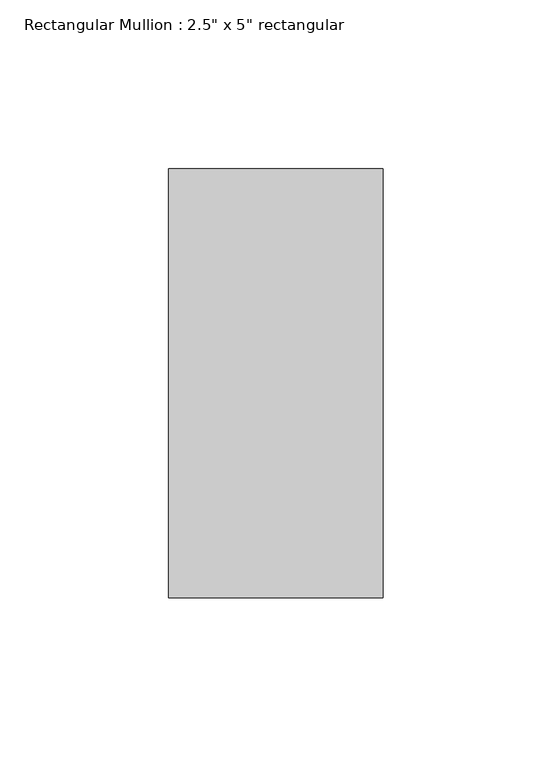
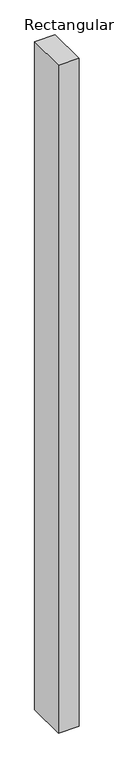
"""IFC4 building model written with IfcOpenShell, lengths in millimetres: member geometry."""

from ifc_helpers import new_model, si_unit, frame, origin, place, context, project, spatial, polyline, outline, extrude, source, transform, mapped, element, save


def member_1ab8d6f1(model_context):
    return source(origin(), model_context, "Body", "SweptSolid", [
        extrude(outline(polyline([(0.0, 63.5), (0.0, -63.5), (-63.5, -63.5), (-63.5, 63.5), (0.0, 63.5)])), frame((0.0, 0.0, -2184.4), z_axis=(0.0, 0.0, 1.0), x_axis=(1.0, 0.0, 0.0)), (0.0, 0.0, 1.0), 2184.4),
    ])


if __name__ == "__main__":
    model = new_model("IFC4")
    model_context = context("Model", 3, world=origin())
    ifc_project = project(units=[si_unit("LENGTHUNIT", "METRE", prefix="MILLI")], contexts=[model_context])
    site = spatial("IfcSite", under=ifc_project)
    building = spatial("IfcBuilding", under=site)
    placement = place(None, origin())
    member_shape = member_1ab8d6f1(model_context)
    element("IfcMember", 1, ObjectType="Rectangular Mullion : 2.5\" x 5\" rectangular", at=placement, inside=building, context=model_context, shape_type="MappedRepresentation", body=[
        mapped(member_shape, transform((0.0, 0.0, 0.0), x_axis=(1.0, 0.0, 0.0), y_axis=(0.0, 1.0, 0.0), z_axis=(0.0, 0.0, 1.0))),
    ])
    save(model, "model.ifc")

# Revit data of these elements
# Type "Rectangular Mullion : 2.5\" x 5\" rectangular"
#   built-in parameter 1007304 = 0.416667 (stored number, unit not read)
#   built-in parameter 1007301 = 0.104167 (stored number, unit not read)
#   built-in parameter 1007300 = 0.104167 (stored number, unit not read)
